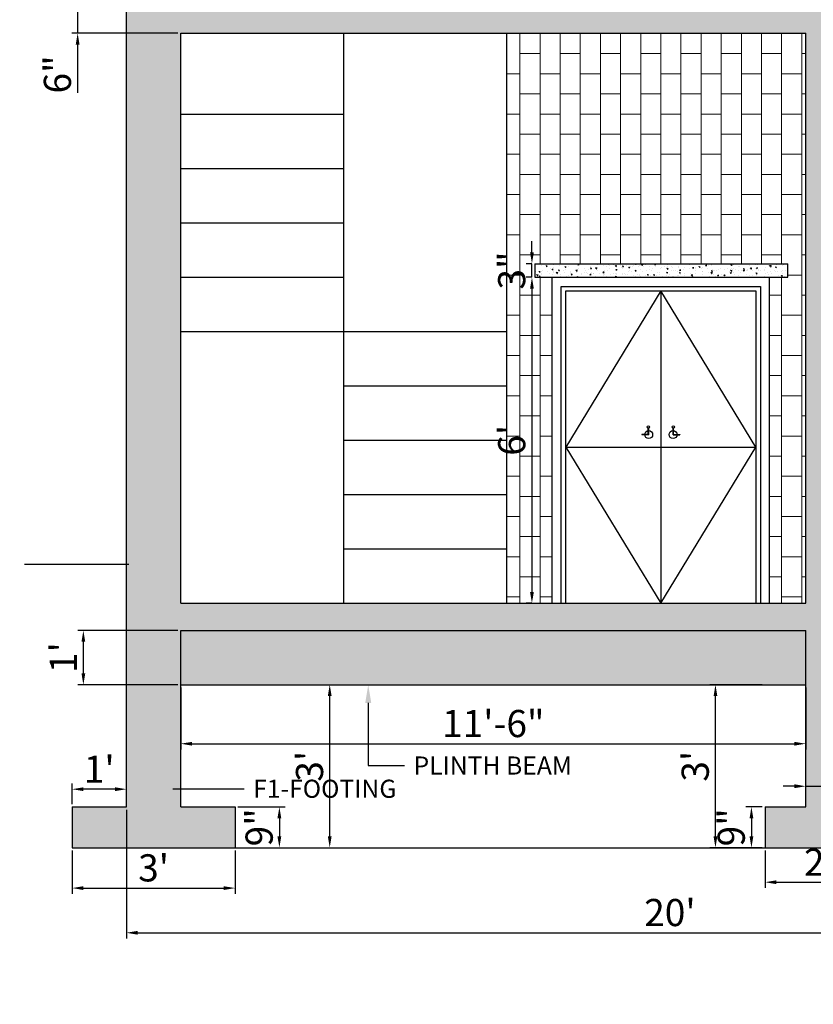
# Model space of a CAD drawing. Units: millimetres. Extents: x 20768 to 23556, y 50760 to 52704.
# Tile 3 of 36: x 20949 to 21124, y 51066 to 51283. Entities that reach past the tile are written whole.
import ezdxf
from ezdxf import colors
from ezdxf.entities.mleader import LeaderData, LeaderLine
from ezdxf.math import Vec2, Vec3

# ---------------------------------------------------------------- set-up
doc = ezdxf.new("R2010")
doc.units = ezdxf.units.MM
for name, color, linetype, lineweight in [('A-ANNO-DIMS', 2, 'Continuous', 18), ('A-ANNO-TEXT', 7, 'Continuous', 18), ('A-ELEV', 7, 'Continuous', 25), ('A-ELEV-PATT', 8, 'Continuous', 13), ('S-ANNO-DIMS', 2, 'Continuous', 18)]:
    doc.layers.add(name, color=color, linetype=linetype, lineweight=lineweight)
doc.styles.get("Standard").update_dxf_attribs({"font": 'arial.ttf'})
doc.dimstyles.new('ISO-25', dxfattribs={"dimtxt": 6, "dimasz": 2.5, "dimexe": 1.25, "dimexo": 0.625, "dimtad": 1, "dimdec": 0, "dimlunit": 3, "dimtxsty": 'Standard', "dimcen": 2.5, "dimadec": 0, "dimazin": 0, "dimtfac": 1, "dimtdec": 0, "dimtmove": 0, "dimatfit": 3, "dimfxl": 1, "dimarcsym": 0})
pattern_1 = [(140, (105.777, 340.6355), (0.23908628, 2.732770035), [0.28575, -3.14325]), (85, (105.777, 340.6355), (-2.86585268, -0.52865132), [0.2286, -2.51460876]), (190.4514447, (105.797, 340.8633), (-2.62676628, 2.20411871), [0.24285013, -2.67135367]), (136.1842, (105.015, 340.6355), (0.63063492, 4.06618561), [0.428625, -4.714875]), (186.635558, (105.0677, 340.9744), (-3.71139187, 3.561062), [0.36427535, -4.00703412]), (81.184151, (105.015, 340.6355), (-3.71139187, 3.561062), [0.3428995, -3.77189598]), (111, (105.2056, 341.0165), (1.53397797, 2.27421587), [0.28575, -3.14325]), (56, (105.2056, 341.0165), (-2.76281949, 0.92703043), [0.2286, -2.5146]), (161.451445, (105.3334, 341.206), (-1.22884153, 3.20124629), [0.24285013, -2.67134906]), (127.5, (105.7771, 340.6355), (-1.268325583, 0.046329049), [0, -2.48412, 0, -2.5527, 0, -2.524125]), (97.5, (105.7771, 340.6355), (-1.502708622, 1.002294938), [0, -1.45542, 0, -2.42697, 0, -0.962025]), (57.5, (105.7771, 339.7859), (0.08593116, 2.033858928), [0, -0.9525, 0, -2.9718, 0, -3.94335]), (47.5, (105.7771, 339.4049), (-0.381397365, 2.22193772), [0, -1.23825, 0, -1.97358, 0, -2.80035])]

# ---------------------------------------------------------------- blocks, each defined once
blk = doc.blocks.new('*D130')
at = {"layer": 'A-ANNO-DIMS', "color": 0, "lineweight": -2, "transparency": 16777216}
for p, q in [((20984.63, 51135.87), (20984.63, 51122.22)), ((21122.63, 51135.87), (21122.63, 51122.22)), ((20987.13, 51123.47), (21120.13, 51123.47))]:
    blk.add_line(p, q, dxfattribs=at)
at = {"layer": 'A-ANNO-DIMS', "color": 0, "transparency": 16777216}
for points in [[(20987.13, 51123.88), (20987.13, 51123.05), (20984.63, 51123.47)], [(21120.13, 51123.88), (21120.13, 51123.05), (21122.63, 51123.47)]]:
    blk.add_solid(points, dxfattribs=at)
at = {"layer": 'Defpoints', "color": 0, "transparency": 16777216}
for p in [(20984.63, 51136.5), (21122.63, 51136.5), (21122.63, 51123.47)]:
    blk.add_point(p, dxfattribs=at)
at = {"layer": 'A-ANNO-DIMS', "color": 0, "transparency": 16777216, "insert": (21053.63, 51127.15), "char_height": 6, "attachment_point": 5}
blk.add_mtext('11\'-6"', dxfattribs=at)
blk = doc.blocks.new('*D131')
at = {"layer": 'A-ANNO-DIMS', "color": 0, "lineweight": -2, "transparency": 16777216}
for p, q in [((20960.63, 51099.87), (20960.63, 51090.33)), ((20996.63, 51099.87), (20996.63, 51090.33)), ((20963.13, 51091.58), (20994.13, 51091.58))]:
    blk.add_line(p, q, dxfattribs=at)
at = {"layer": 'A-ANNO-DIMS', "color": 0, "transparency": 16777216}
for points in [[(20963.13, 51091.99), (20963.13, 51091.16), (20960.63, 51091.58)], [(20994.13, 51091.99), (20994.13, 51091.16), (20996.63, 51091.58)]]:
    blk.add_solid(points, dxfattribs=at)
at = {"layer": 'Defpoints', "color": 0, "transparency": 16777216}
for p in [(20960.63, 51100.5), (20996.63, 51100.5), (20996.63, 51091.58)]:
    blk.add_point(p, dxfattribs=at)
at = {"layer": 'A-ANNO-DIMS', "color": 0, "transparency": 16777216, "insert": (20978.63, 51095.27), "char_height": 6, "attachment_point": 5}
blk.add_mtext("3'", dxfattribs=at)
blk = doc.blocks.new('*D132')
at = {"layer": 'A-ANNO-DIMS', "color": 0, "lineweight": -2, "transparency": 16777216}
for p, q in [((20997.26, 51109.5), (21007.65, 51109.5)), ((21006.4, 51107), (21006.4, 51103)), ((20997.26, 51100.5), (21007.65, 51100.5))]:
    blk.add_line(p, q, dxfattribs=at)
at = {"layer": 'A-ANNO-DIMS', "color": 0, "transparency": 16777216}
for points in [[(21005.98, 51107), (21006.82, 51107), (21006.4, 51109.5)], [(21005.98, 51103), (21006.82, 51103), (21006.4, 51100.5)]]:
    blk.add_solid(points, dxfattribs=at)
at = {"layer": 'Defpoints', "color": 0, "transparency": 16777216}
for p in [(20996.63, 51109.5), (20996.63, 51100.5), (21006.4, 51100.5)]:
    blk.add_point(p, dxfattribs=at)
at = {"layer": 'A-ANNO-DIMS', "color": 0, "transparency": 16777216, "insert": (21002.71, 51105), "char_height": 6, "attachment_point": 5, "rotation": 90}
blk.add_mtext('9"', dxfattribs=at)
blk = doc.blocks.new('*D133')
at = {"layer": 'A-ANNO-DIMS', "color": 0, "lineweight": -2, "transparency": 16777216}
for p, q in [((20960.63, 51110.12), (20960.63, 51114.67)), ((20972.63, 51110.12), (20972.63, 51114.67)), ((20970.13, 51113.42), (20963.13, 51113.42))]:
    blk.add_line(p, q, dxfattribs=at)
at = {"layer": 'A-ANNO-DIMS', "color": 0, "transparency": 16777216}
for points in [[(20963.13, 51113.84), (20963.13, 51113.01), (20960.63, 51113.42)], [(20970.13, 51113.84), (20970.13, 51113.01), (20972.63, 51113.42)]]:
    blk.add_solid(points, dxfattribs=at)
at = {"layer": 'Defpoints', "color": 0, "transparency": 16777216}
for p in [(20960.63, 51113.42), (20960.63, 51109.5), (20972.63, 51109.5)]:
    blk.add_point(p, dxfattribs=at)
at = {"layer": 'A-ANNO-DIMS', "color": 0, "transparency": 16777216, "insert": (20966.63, 51117.06), "char_height": 6, "attachment_point": 5}
blk.add_mtext("1'", dxfattribs=at)
blk = doc.blocks.new('*D135')
at = {"layer": 'A-ANNO-DIMS', "color": 0, "lineweight": -2, "transparency": 16777216}
for p, q in [((21122.63, 51110.12), (21122.63, 51115.33)), ((21128.63, 51110.12), (21128.63, 51115.33)), ((21120.13, 51114.08), (21117.63, 51114.08)), ((21122.63, 51114.08), (21128.63, 51114.08)), ((21131.13, 51114.08), (21141.81, 51114.08))]:
    blk.add_line(p, q, dxfattribs=at)
at = {"layer": 'A-ANNO-DIMS', "color": 0, "transparency": 16777216}
for points in [[(21120.13, 51114.5), (21120.13, 51113.66), (21122.63, 51114.08)], [(21131.13, 51114.5), (21131.13, 51113.66), (21128.63, 51114.08)]]:
    blk.add_solid(points, dxfattribs=at)
at = {"layer": 'Defpoints', "color": 0, "transparency": 16777216}
for p in [(21128.63, 51114.08), (21122.63, 51109.5), (21128.63, 51109.5)]:
    blk.add_point(p, dxfattribs=at)
at = {"layer": 'A-ANNO-DIMS', "color": 0, "transparency": 16777216, "insert": (21137.72, 51117.77), "char_height": 6, "attachment_point": 5}
blk.add_mtext('6"', dxfattribs=at)
blk = doc.blocks.new('*D136')
at = {"layer": 'A-ANNO-DIMS', "color": 0, "lineweight": -2, "transparency": 16777216}
for p, q in [((21113.63, 51099.87), (21113.63, 51091.63)), ((21137.63, 51099.87), (21137.63, 51091.63)), ((21116.13, 51092.88), (21135.13, 51092.88))]:
    blk.add_line(p, q, dxfattribs=at)
at = {"layer": 'A-ANNO-DIMS', "color": 0, "transparency": 16777216}
for points in [[(21116.13, 51093.29), (21116.13, 51092.46), (21113.63, 51092.88)], [(21135.13, 51093.29), (21135.13, 51092.46), (21137.63, 51092.88)]]:
    blk.add_solid(points, dxfattribs=at)
at = {"layer": 'Defpoints', "color": 0, "transparency": 16777216}
for p in [(21113.63, 51100.5), (21137.63, 51100.5), (21137.63, 51092.88)]:
    blk.add_point(p, dxfattribs=at)
at = {"layer": 'A-ANNO-DIMS', "color": 0, "transparency": 16777216, "insert": (21125.63, 51096.52), "char_height": 6, "attachment_point": 5}
blk.add_mtext("2'", dxfattribs=at)
blk = doc.blocks.new('*D137')
at = {"layer": 'A-ANNO-DIMS', "color": 0, "lineweight": -2, "transparency": 16777216}
for p, q in [((21113.01, 51109.5), (21109.37, 51109.5)), ((21110.62, 51107), (21110.62, 51103)), ((21113.01, 51100.5), (21109.37, 51100.5))]:
    blk.add_line(p, q, dxfattribs=at)
at = {"layer": 'A-ANNO-DIMS', "color": 0, "transparency": 16777216}
for points in [[(21110.21, 51107), (21111.04, 51107), (21110.62, 51109.5)], [(21110.21, 51103), (21111.04, 51103), (21110.62, 51100.5)]]:
    blk.add_solid(points, dxfattribs=at)
at = {"layer": 'Defpoints', "color": 0, "transparency": 16777216}
for p in [(21113.63, 51109.5), (21110.62, 51100.5), (21113.63, 51100.5)]:
    blk.add_point(p, dxfattribs=at)
at = {"layer": 'A-ANNO-DIMS', "color": 0, "transparency": 16777216, "insert": (21106.94, 51105), "char_height": 6, "attachment_point": 5, "rotation": 90}
blk.add_mtext('9"', dxfattribs=at)
blk = doc.blocks.new('*D112')
at = {"layer": 'A-ANNO-DIMS', "color": 0, "lineweight": -2, "transparency": 16777216}
for p, q in [((20997.26, 51136.5), (21018.77, 51136.5)), ((21017.52, 51103), (21017.52, 51134)), ((20997.26, 51100.5), (21018.77, 51100.5))]:
    blk.add_line(p, q, dxfattribs=at)
at = {"layer": 'A-ANNO-DIMS', "color": 0, "transparency": 16777216}
for points in [[(21017.1, 51134), (21017.93, 51134), (21017.52, 51136.5)], [(21017.1, 51103), (21017.93, 51103), (21017.52, 51100.5)]]:
    blk.add_solid(points, dxfattribs=at)
at = {"layer": 'Defpoints', "color": 0, "transparency": 16777216}
for p in [(20996.63, 51136.5), (21017.52, 51136.5), (20996.63, 51100.5)]:
    blk.add_point(p, dxfattribs=at)
at = {"layer": 'A-ANNO-DIMS', "color": 0, "transparency": 16777216, "insert": (21013.83, 51118.5), "char_height": 6, "attachment_point": 5, "rotation": 90}
blk.add_mtext("3'", dxfattribs=at)
blk = doc.blocks.new('*D115')
at = {"layer": 'A-ANNO-DIMS', "color": 0, "lineweight": -2, "transparency": 16777216}
for p, q in [((20961.86, 51288.9), (20961.86, 51291.4)), ((20984.01, 51286.4), (20960.61, 51286.4)), ((20961.86, 51286.4), (20961.86, 51280.4)), ((20984.01, 51280.4), (20960.61, 51280.4)), ((20961.86, 51277.9), (20961.86, 51267.22))]:
    blk.add_line(p, q, dxfattribs=at)
at = {"layer": 'A-ANNO-DIMS', "color": 0, "transparency": 16777216}
for points in [[(20961.44, 51288.9), (20962.28, 51288.9), (20961.86, 51286.4)], [(20961.44, 51277.9), (20962.28, 51277.9), (20961.86, 51280.4)]]:
    blk.add_solid(points, dxfattribs=at)
at = {"layer": 'Defpoints', "color": 0, "transparency": 16777216}
for p in [(20984.63, 51286.4), (20961.86, 51280.4), (20984.63, 51280.4)]:
    blk.add_point(p, dxfattribs=at)
at = {"layer": 'A-ANNO-DIMS', "color": 0, "transparency": 16777216, "insert": (20958.17, 51271.31), "char_height": 6, "attachment_point": 5, "rotation": 90}
blk.add_mtext('6"', dxfattribs=at)
blk = doc.blocks.new('*D124')
at = {"layer": 'A-ANNO-DIMS', "color": 0, "lineweight": -2, "transparency": 16777216}
for p, q in [((21062.17, 51226.5), (21060.91, 51226.5)), ((21062.16, 51224), (21062.16, 51157)), ((21062.17, 51154.5), (21060.91, 51154.5))]:
    blk.add_line(p, q, dxfattribs=at)
at = {"layer": 'A-ANNO-DIMS', "color": 0, "transparency": 16777216}
for points in [[(21061.75, 51224), (21062.58, 51224), (21062.16, 51226.5)], [(21061.75, 51157), (21062.58, 51157), (21062.16, 51154.5)]]:
    blk.add_solid(points, dxfattribs=at)
at = {"layer": 'Defpoints', "color": 0, "transparency": 16777216}
for p in [(21062.79, 51226.5), (21062.16, 51154.5), (21062.79, 51154.5)]:
    blk.add_point(p, dxfattribs=at)
at = {"layer": 'A-ANNO-DIMS', "color": 0, "transparency": 16777216, "insert": (21058.48, 51190.5), "char_height": 6, "attachment_point": 5, "rotation": 90}
blk.add_mtext("6'", dxfattribs=at)
blk = doc.blocks.new('*D125')
at = {"layer": 'A-ANNO-DIMS', "color": 0, "lineweight": -2, "transparency": 16777216}
for p, q in [((21062.16, 51232), (21062.16, 51234.5)), ((21062.17, 51229.5), (21060.91, 51229.5)), ((21062.16, 51226.5), (21062.16, 51229.5)), ((21062.17, 51226.5), (21060.91, 51226.5)), ((21062.16, 51224), (21062.16, 51221.5))]:
    blk.add_line(p, q, dxfattribs=at)
at = {"layer": 'A-ANNO-DIMS', "color": 0, "transparency": 16777216}
for points in [[(21061.75, 51232), (21062.58, 51232), (21062.16, 51229.5)], [(21061.75, 51224), (21062.58, 51224), (21062.16, 51226.5)]]:
    blk.add_solid(points, dxfattribs=at)
at = {"layer": 'Defpoints', "color": 0, "transparency": 16777216}
for p in [(21062.16, 51229.5), (21062.79, 51229.5), (21062.79, 51226.5)]:
    blk.add_point(p, dxfattribs=at)
at = {"layer": 'A-ANNO-DIMS', "color": 0, "transparency": 16777216, "insert": (21058.47, 51228), "char_height": 6, "attachment_point": 5, "rotation": 90}
blk.add_mtext('3"', dxfattribs=at)
blk = doc.blocks.new('*D126')
at = {"layer": 'A-ANNO-DIMS', "color": 0, "lineweight": -2, "transparency": 16777216}
for p, q in [((20984.01, 51148.5), (20961.87, 51148.5)), ((20963.12, 51139), (20963.12, 51146)), ((20984.01, 51136.5), (20961.87, 51136.5))]:
    blk.add_line(p, q, dxfattribs=at)
at = {"layer": 'A-ANNO-DIMS', "color": 0, "transparency": 16777216}
for points in [[(20962.71, 51146), (20963.54, 51146), (20963.12, 51148.5)], [(20962.71, 51139), (20963.54, 51139), (20963.12, 51136.5)]]:
    blk.add_solid(points, dxfattribs=at)
at = {"layer": 'Defpoints', "color": 0, "transparency": 16777216}
for p in [(20963.12, 51148.5), (20984.63, 51148.5), (20984.63, 51136.5)]:
    blk.add_point(p, dxfattribs=at)
at = {"layer": 'A-ANNO-DIMS', "color": 0, "transparency": 16777216, "insert": (20959.49, 51142.5), "char_height": 6, "attachment_point": 5, "rotation": 90}
blk.add_mtext("1'", dxfattribs=at)
blk = doc.blocks.new('*D128')
at = {"layer": 'A-ANNO-DIMS', "color": 0, "lineweight": -2, "transparency": 16777216}
for p, q in [((21113.01, 51136.5), (21101.43, 51136.5)), ((21102.68, 51103), (21102.68, 51134)), ((21113.01, 51100.5), (21101.43, 51100.5))]:
    blk.add_line(p, q, dxfattribs=at)
at = {"layer": 'A-ANNO-DIMS', "color": 0, "transparency": 16777216}
for points in [[(21102.27, 51134), (21103.1, 51134), (21102.68, 51136.5)], [(21102.27, 51103), (21103.1, 51103), (21102.68, 51100.5)]]:
    blk.add_solid(points, dxfattribs=at)
at = {"layer": 'Defpoints', "color": 0, "transparency": 16777216}
for p in [(21102.68, 51136.5), (21113.63, 51136.5), (21113.63, 51100.5)]:
    blk.add_point(p, dxfattribs=at)
at = {"layer": 'A-ANNO-DIMS', "color": 0, "transparency": 16777216, "insert": (21098.99, 51118.5), "char_height": 6, "attachment_point": 5, "rotation": 90}
blk.add_mtext("3'", dxfattribs=at)
blk = doc.blocks.new('*D111')
at = {"layer": 'A-ANNO-DIMS', "color": 0, "lineweight": -2, "transparency": 16777216}
for p, q in [((20972.63, 51108.87), (20972.63, 51080.46)), ((21212.63, 51108.87), (21212.63, 51080.46)), ((20975.13, 51081.71), (21210.13, 51081.71))]:
    blk.add_line(p, q, dxfattribs=at)
at = {"layer": 'A-ANNO-DIMS', "color": 0, "transparency": 16777216}
for points in [[(20975.13, 51082.13), (20975.13, 51081.29), (20972.63, 51081.71)], [(21210.13, 51082.13), (21210.13, 51081.29), (21212.63, 51081.71)]]:
    blk.add_solid(points, dxfattribs=at)
at = {"layer": 'Defpoints', "color": 0, "transparency": 16777216}
for p in [(20972.63, 51109.5), (21212.63, 51109.5), (21212.63, 51081.71)]:
    blk.add_point(p, dxfattribs=at)
at = {"layer": 'A-ANNO-DIMS', "color": 0, "transparency": 16777216, "insert": (21092.63, 51085.4), "char_height": 6, "attachment_point": 5}
blk.add_mtext("20'", dxfattribs=at)
blk = doc.blocks.new('*D229')
at = {"layer": 'Defpoints', "color": 0, "transparency": 16777216}
for p in [(20963.6, 51532.3), (20960.63, 51100.5), (21253.63, 51100.5)]:
    blk.add_point(p, dxfattribs=at)
at = {"layer": 'S-ANNO-DIMS', "color": 0, "lineweight": -2, "transparency": 16777216}
for p, q in [((20964.22, 51532.3), (21254.88, 51532.3)), ((21253.63, 51529.8), (21253.63, 51103)), ((20961.26, 51100.5), (21254.88, 51100.5))]:
    blk.add_line(p, q, dxfattribs=at)
at = {"layer": 'S-ANNO-DIMS', "color": 0, "transparency": 16777216}
for points in [[(21253.22, 51529.8), (21254.05, 51529.8), (21253.63, 51532.3)], [(21253.22, 51103), (21254.05, 51103), (21253.63, 51100.5)]]:
    blk.add_solid(points, dxfattribs=at)
at = {"layer": 'S-ANNO-DIMS', "color": 0, "transparency": 16777216, "insert": (21249.94, 51316.4), "char_height": 6, "attachment_point": 5, "rotation": 90}
blk.add_mtext('36\'-0"', dxfattribs=at)

msp = doc.modelspace()

# ---------------------------------------------------------------- hatches: boundary and pattern name
at = {"layer": 'A-ELEV-PATT'}
h = msp.add_hatch(dxfattribs=at)
h.set_pattern_fill('AR-CONC', color=256, scale=0.015, angle=90)
h.set_pattern_definition(pattern_1)
h.paths.add_polyline_path([(21212.63, 51490.3), (21200.63, 51490.3), (21200.63, 51418.3), (21128.63, 51418.3), (21128.63, 51490.3), (21122.63, 51490.3), (21122.63, 51418.3), (20972.63, 51418.3), (20972.63, 51109.5), (20960.63, 51109.5), (20960.63, 51100.5), (20996.63, 51100.5), (20996.63, 51109.5), (20984.63, 51109.5), (20984.63, 51148.5), (21122.63, 51148.5), (21122.63, 51109.5), (21113.63, 51109.5), (21113.63, 51100.5), (21137.63, 51100.5), (21137.63, 51109.5), (21128.63, 51109.5), (21128.63, 51148.5), (21212.63, 51148.5)])
h.paths.add_polyline_path([(21122.63, 51280.4), (21122.63, 51154.5), (20984.63, 51154.5), (20984.63, 51280.4)], flags=16)
h.paths.add_polyline_path([(21122.63, 51286.4), (20984.63, 51286.4), (20984.63, 51412.3), (21122.63, 51412.3)], flags=16)
h.paths.add_polyline_path([(21128.63, 51280.4), (21200.63, 51280.4), (21200.63, 51154.5), (21128.63, 51154.5)], flags=16)
h.paths.add_polyline_path([(21128.63, 51286.4), (21128.63, 51412.3), (21200.63, 51412.3), (21200.63, 51286.4)], flags=16)
h.paths.add_polyline_path([(21062.79, 51358.4), (21062.79, 51361.4), (21118.63, 51361.4), (21118.63, 51358.4)], flags=0)
h.paths.add_polyline_path([(21111.63, 51320.9), (21090.63, 51286.4), (21069.63, 51320.9), (21069.63, 51355.4), (21111.63, 51355.4)], flags=0)
h.paths.add_polyline_path([(21069.63, 51320.9), (21090.63, 51355.4), (21111.63, 51320.9)], flags=0)
h.paths.add_polyline_path([(21136.63, 51320.9), (21136.63, 51368), (21167.33, 51368), (21167.33, 51320.9)], flags=0)
h.paths.add_polyline_path([(21138.63, 51322.9), (21138.63, 51350.9), (21165.33, 51350.9), (21165.33, 51322.9)], flags=0)
h.paths.add_polyline_path([(21140.63, 51324.9), (21140.63, 51348.9), (21150.98, 51348.9), (21150.98, 51324.9)], flags=0)
h.paths.add_polyline_path([(21136.63, 51236.1), (21167.33, 51236.1), (21167.33, 51189), (21136.63, 51189)], flags=0)
h.paths.add_polyline_path([(21152.98, 51324.9), (21152.98, 51348.9), (21163.33, 51348.9), (21163.33, 51324.9)], flags=0)
h.paths.add_polyline_path([(21094.84, 51323.58), (21094.21, 51323.58, -0.960515), (21092.46, 51323.65, -0.414214), (21093.33, 51324.52), (21093.33, 51325.09, -0.357901), (21093.11, 51325.35, -1), (21093.66, 51325.35, -0.34824), (21093.45, 51325.09), (21093.45, 51324.51, -0.376216), (21094.21, 51323.65), (21094.84, 51323.65)], flags=0)
h.paths.add_polyline_path([(21138.63, 51234.1), (21165.33, 51234.1), (21165.33, 51221), (21138.63, 51221)], flags=0)
h.paths.add_polyline_path([(21118.63, 51229.5), (21118.63, 51226.5), (21062.79, 51226.5), (21062.79, 51229.5)], flags=0)
h.paths.add_polyline_path([(21087.06, 51323.58), (21086.42, 51323.58), (21086.42, 51323.65), (21087.06, 51323.65, -0.376216), (21087.82, 51324.51), (21087.82, 51325.09, -0.34824), (21087.61, 51325.35, -1), (21088.15, 51325.35, -0.357901), (21087.94, 51325.09), (21087.94, 51324.52, -0.414214), (21088.81, 51323.65, -0.960515)], flags=0)
h.paths.add_polyline_path([(21111.63, 51223.5), (21111.63, 51189), (21090.63, 51154.5), (21069.63, 51189), (21069.63, 51223.5)], flags=0)
h.paths.add_polyline_path([(21138.63, 51219), (21165.33, 51219), (21165.33, 51191), (21138.63, 51191)], flags=0)
h.paths.add_polyline_path([(21140.63, 51217), (21150.98, 51217), (21150.98, 51193), (21140.63, 51193)], flags=0)
h.paths.add_polyline_path([(21056.63, 51166.5), (21020.63, 51166.5), (21020.63, 51214.5), (21056.63, 51214.5)], flags=0)
h.paths.add_polyline_path([(21056.63, 51298.4), (21020.63, 51298.4), (21020.63, 51346.4), (21056.63, 51346.4)], flags=0)
h.paths.add_polyline_path([(21090.63, 51223.5), (21111.63, 51189), (21069.63, 51189)], flags=0)
h.paths.add_polyline_path([(21138.63, 51352.9), (21138.63, 51366), (21165.33, 51366), (21165.33, 51352.9)], flags=0)
h.paths.add_polyline_path([(21152.98, 51217), (21163.33, 51217), (21163.33, 51193), (21152.98, 51193)], flags=0)
h.paths.add_polyline_path([(21093.66, 51193.45, -0.34824), (21093.45, 51193.19), (21093.45, 51192.61, -0.376216), (21094.21, 51191.75), (21094.84, 51191.75), (21094.84, 51191.68), (21094.21, 51191.68, -0.960515), (21092.46, 51191.75, -0.414214), (21093.33, 51192.62), (21093.33, 51193.19, -0.357901), (21093.11, 51193.45, -1)], flags=0)
h.paths.add_polyline_path([(21088.15, 51193.45, -0.357901), (21087.94, 51193.19), (21087.94, 51192.62, -0.414214), (21088.81, 51191.75, -0.960515), (21087.06, 51191.68), (21086.42, 51191.68), (21086.42, 51191.75), (21087.06, 51191.75, -0.376216), (21087.82, 51192.61), (21087.82, 51193.19, -0.34824), (21087.61, 51193.45, -1)], flags=0)
h = msp.add_hatch(dxfattribs=at)
h.set_pattern_fill('BRICK', color=256, scale=0.7, angle=90)
h.set_pattern_definition([(90, (105.777, 340.6355), (-4.445, 3e-16), []), (180, (105.777, 340.6355), (-1e-15, -8.89), [4.445, -4.445]), (180, (105.777, 345.0805), (-1e-15, -8.89), [-4.445, 4.445])])
h.paths.add_polyline_path([(21122.63, 51280.4), (21056.63, 51280.4), (21056.63, 51154.5), (21066.63, 51154.5), (21066.63, 51226.5), (21062.79, 51226.5), (21062.79, 51229.5), (21118.63, 51229.5), (21118.63, 51226.5), (21114.63, 51226.5), (21114.63, 51154.5), (21122.63, 51154.5)])
h = msp.add_hatch(dxfattribs=at)
h.set_pattern_fill('AR-CONC', color=256, scale=0.015, angle=90)
h.paths.add_polyline_path([(21118.63, 51229.5), (21062.79, 51229.5), (21062.79, 51226.5), (21118.63, 51226.5)])
h = msp.add_hatch(dxfattribs=at)
h.set_pattern_fill('AR-CONC', color=256, scale=8)
h.paths.add_polyline_path([(21106.86, 51149.66), (21094.86, 51149.66), (21094.86, 51077.66), (21022.86, 51077.66), (21022.86, 51149.66), (21016.86, 51149.66), (21016.86, 51077.66), (20866.86, 51077.66), (20866.86, 50768.86), (20854.86, 50768.86), (20854.86, 50759.86), (20890.86, 50759.86), (20890.86, 50768.86), (20878.86, 50768.86), (20878.86, 50807.86), (21016.86, 50807.86), (21016.86, 50768.86), (21007.86, 50768.86), (21007.86, 50759.86), (21031.86, 50759.86), (21031.86, 50768.86), (21022.86, 50768.86), (21022.86, 50807.86), (21094.86, 50807.86), (21094.86, 50768.86), (21082.86, 50768.86), (21082.86, 50759.86), (21118.86, 50759.86), (21118.86, 50768.86), (21106.86, 50768.86)])
h.paths.add_polyline_path([(21022.86, 50939.76), (21094.86, 50939.76), (21094.86, 50813.86), (21022.86, 50813.86)], flags=16)
h.paths.add_polyline_path([(21016.86, 50939.76), (21016.86, 50813.86), (20878.86, 50813.86), (20878.86, 50939.76)], flags=16)
h.paths.add_polyline_path([(21022.86, 50945.76), (21022.86, 51071.66), (21094.86, 51071.66), (21094.86, 50945.76)], flags=16)
h.paths.add_polyline_path([(21016.86, 50945.76), (20878.86, 50945.76), (20878.86, 51071.66), (21016.86, 51071.66)], flags=16)
h.paths.add_polyline_path([(20957.01, 51017.76), (20957.01, 51020.76), (21012.86, 51020.76), (21012.86, 51017.76)], flags=0)
h.paths.add_polyline_path([(21005.86, 50980.26), (20984.86, 50945.76), (20963.86, 50980.26), (20963.86, 51014.76), (21005.86, 51014.76)], flags=0)
h.paths.add_polyline_path([(20963.86, 50980.26), (20984.86, 51014.76), (21005.86, 50980.26)], flags=0)
h.paths.add_polyline_path([(21030.86, 50980.26), (21030.86, 51027.36), (21061.56, 51027.36), (21061.56, 50980.26)], flags=0)
h.paths.add_polyline_path([(21032.86, 50982.26), (21032.86, 51010.26), (21059.56, 51010.26), (21059.56, 50982.26)], flags=0)
h.paths.add_polyline_path([(21034.86, 50984.26), (21034.86, 51008.26), (21045.21, 51008.26), (21045.21, 50984.26)], flags=0)
h.paths.add_polyline_path([(21030.86, 50895.46), (21061.56, 50895.46), (21061.56, 50848.36), (21030.86, 50848.36)], flags=0)
h.paths.add_polyline_path([(21032.86, 50893.46), (21059.56, 50893.46), (21059.56, 50880.36), (21032.86, 50880.36)], flags=0)
h.paths.add_polyline_path([(21047.21, 50984.26), (21047.21, 51008.26), (21057.56, 51008.26), (21057.56, 50984.26)], flags=0)
h.paths.add_polyline_path([(20989.07, 50982.94), (20988.43, 50982.94, -0.960515), (20986.68, 50983.01, -0.414214), (20987.56, 50983.89), (20987.56, 50984.45, -0.357901), (20987.34, 50984.72, -1), (20987.88, 50984.72, -0.34824), (20987.67, 50984.45), (20987.67, 50983.88, -0.376216), (20988.43, 50983.01), (20989.07, 50983.01)], flags=0)
h.paths.add_polyline_path([(21012.86, 50888.86), (21012.86, 50885.86), (20957.01, 50885.86), (20957.01, 50888.86)], flags=0)
h.paths.add_polyline_path([(20981.29, 50982.94), (20980.65, 50982.94), (20980.65, 50983.01), (20981.28, 50983.01, -0.376216), (20982.04, 50983.88), (20982.04, 50984.45, -0.34824), (20981.83, 50984.72, -1), (20982.38, 50984.72, -0.357901), (20982.16, 50984.45), (20982.16, 50983.89, -0.414214), (20983.04, 50983.01, -0.960515)], flags=0)
h.paths.add_polyline_path([(21005.86, 50882.86), (21005.86, 50848.36), (20984.86, 50813.86), (20963.86, 50848.36), (20963.86, 50882.86)], flags=0)
h.paths.add_polyline_path([(21032.86, 50878.36), (21059.56, 50878.36), (21059.56, 50850.36), (21032.86, 50850.36)], flags=0)
h.paths.add_polyline_path([(21034.86, 50876.36), (21045.21, 50876.36), (21045.21, 50852.36), (21034.86, 50852.36)], flags=0)
h.paths.add_polyline_path([(20984.86, 50882.86), (21005.86, 50848.36), (20963.86, 50848.36)], flags=0)
h.paths.add_polyline_path([(20950.86, 50825.86), (20914.86, 50825.86), (20914.86, 50873.86), (20950.86, 50873.86)], flags=0)
h.paths.add_polyline_path([(20950.86, 50957.76), (20914.86, 50957.76), (20914.86, 51005.76), (20950.86, 51005.76)], flags=0)
h.paths.add_polyline_path([(21047.21, 50876.36), (21057.56, 50876.36), (21057.56, 50852.36), (21047.21, 50852.36)], flags=0)
h.paths.add_polyline_path([(21032.86, 51012.26), (21032.86, 51025.36), (21059.56, 51025.36), (21059.56, 51012.26)], flags=0)
h.paths.add_polyline_path([(20987.88, 50852.82, -0.34824), (20987.67, 50852.55), (20987.67, 50851.98, -0.376216), (20988.43, 50851.11), (20989.07, 50851.11), (20989.07, 50851.04), (20988.43, 50851.04, -0.960515), (20986.68, 50851.11, -0.414214), (20987.56, 50851.99), (20987.56, 50852.55, -0.357901), (20987.34, 50852.82, -1)], flags=0)
h.paths.add_polyline_path([(20982.38, 50852.82, -0.357901), (20982.16, 50852.55), (20982.16, 50851.99, -0.414214), (20983.04, 50851.11, -0.960515), (20981.29, 50851.04), (20980.65, 50851.04), (20980.65, 50851.11), (20981.28, 50851.11, -0.376216), (20982.04, 50851.98), (20982.04, 50852.55, -0.34824), (20981.83, 50852.82, -1)], flags=0)
h = msp.add_hatch(dxfattribs=at)
h.set_pattern_fill('AR-CONC', color=256, scale=0.015, angle=90)
h.set_pattern_definition(pattern_1)
h.paths.add_polyline_path([(21122.63, 51148.5), (20984.63, 51148.5), (20984.63, 51136.5), (21122.63, 51136.5)])

# ---------------------------------------------------------------- linework, layer by layer
at = {"layer": 'A-ELEV'}
for p, q in [((20972.63, 51109.5), (20972.63, 51526.3)), ((20984.63, 51154.5), (20984.63, 51280.4)), ((20984.63, 51280.4), (21122.63, 51280.4)), ((21020.63, 51154.5), (21020.63, 51280.4)), ((21056.63, 51154.5), (21056.63, 51280.4)), ((21122.63, 51154.5), (21122.63, 51280.4)), ((20984.63, 51262.5), (21020.63, 51262.5)), ((20984.63, 51250.5), (21020.63, 51250.5)), ((20984.63, 51238.5), (21020.63, 51238.5)), ((21062.79, 51229.5), (21118.63, 51229.5)), ((21062.79, 51229.5), (21062.79, 51226.5)), ((21118.63, 51226.5), (21118.63, 51229.5)), ((20984.63, 51226.5), (21020.63, 51226.5)), ((21062.79, 51226.5), (21118.63, 51226.5)), ((21066.63, 51154.5), (21066.63, 51226.5)), ((21114.63, 51154.5), (21114.63, 51226.5)), ((21090.63, 51223.5), (21090.63, 51154.5)), ((20984.63, 51214.5), (21056.63, 51214.5)), ((21020.63, 51202.5), (21056.63, 51202.5)), ((21087.82, 51191.75), (21087.82, 51193.19)), ((21087.94, 51191.68), (21087.94, 51193.19)), ((21093.33, 51191.68), (21093.33, 51193.19)), ((21093.45, 51191.75), (21093.45, 51193.19)), ((21087.82, 51191.75), (21086.42, 51191.75)), ((21086.42, 51191.75), (21086.42, 51191.68)), ((21087.94, 51191.68), (21086.42, 51191.68)), ((21093.33, 51191.68), (21094.84, 51191.68)), ((21093.45, 51191.75), (21094.84, 51191.75)), ((21094.84, 51191.75), (21094.84, 51191.68)), ((21020.63, 51190.5), (21056.63, 51190.5)), ((21069.63, 51189), (21111.63, 51189)), ((21020.63, 51178.5), (21056.63, 51178.5)), ((21020.63, 51166.5), (21056.63, 51166.5)), ((20984.63, 51154.5), (21122.63, 51154.5)), ((20984.63, 51109.5), (20984.63, 51148.5)), ((20984.63, 51148.5), (21122.63, 51148.5)), ((21122.63, 51109.5), (21122.63, 51148.5)), ((20984.63, 51136.5), (21122.63, 51136.5)), ((20960.63, 51109.5), (20972.63, 51109.5)), ((20960.63, 51109.5), (20960.63, 51100.5)), ((20984.63, 51109.5), (20996.63, 51109.5)), ((20996.63, 51109.5), (20996.63, 51100.5)), ((21113.63, 51109.5), (21122.63, 51109.5)), ((21113.63, 51109.5), (21113.63, 51100.5)), ((20960.63, 51100.5), (20996.63, 51100.5)), ((21113.63, 51100.5), (21137.63, 51100.5))]:
    msp.add_line(p, q, dxfattribs=at)
for points in [[(21068.63, 51154.5), (21068.63, 51224.5), (21112.63, 51224.5), (21112.63, 51154.5)], [(21069.63, 51154.5), (21069.63, 51223.5), (21111.63, 51223.5), (21111.63, 51154.5)]]:
    msp.add_lwpolyline(points, dxfattribs=at)
msp.add_lwpolyline([(21111.63, 51189), (21090.63, 51223.5), (21069.63, 51189), (21090.63, 51154.5)], close=True, dxfattribs=at)
for centre, radius in [((21087.88, 51193.45), 0.272), ((21093.39, 51193.45), 0.272), ((21087.94, 51191.75), 0.877), ((21093.33, 51191.75), 0.877)]:
    msp.add_circle(centre, radius, dxfattribs=at)

# ---------------------------------------------------------------- dimensions: what is measured, and where the dimension line sits
at = {"layer": 'A-ANNO-DIMS'}
for base, p1, p2, picture, middle in [((20961.86, 51280.4), (20984.63, 51286.4), (20984.63, 51280.4), '*D115', (20958.17, 51271.31)), ((21062.16, 51154.5), (21062.79, 51226.5), (21062.79, 51154.5), '*D124', (21058.48, 51190.5)), ((20963.12, 51148.5), (20984.63, 51136.5), (20984.63, 51148.5), '*D126', (20959.49, 51142.5)), ((21017.52, 51136.5), (20996.63, 51100.5), (20996.63, 51136.5), '*D112', (21013.83, 51118.5)), ((21102.68, 51136.5), (21113.63, 51100.5), (21113.63, 51136.5), '*D128', (21098.99, 51118.5)), ((21006.4, 51100.5), (20996.63, 51109.5), (20996.63, 51100.5), '*D132', (21002.71, 51105)), ((21110.62, 51100.5), (21113.63, 51109.5), (21113.63, 51100.5), '*D137', (21106.94, 51105))]:
    dim = msp.add_linear_dim(base=base, p1=p1, p2=p2, angle=90, dimstyle='ISO-25', override={"dimclrd": 0, "dimclre": 0, "dimclrt": 0}, dxfattribs=at)
    dim.commit()
    dim.dimension.update_dxf_attribs({"geometry": picture, "text_midpoint": middle})
dim = msp.add_linear_dim(base=(21062.16, 51229.5), p1=(21062.79, 51226.5), p2=(21062.79, 51229.5), angle=90, dimstyle='ISO-25', override={"dimclrd": 0, "dimclre": 0, "dimclrt": 0}, dxfattribs=at)
dim.commit()
dim.dimension.update_dxf_attribs({"geometry": '*D125', "text_midpoint": (21062.16, 51228), "dimtype": 160})
for base, p1, p2, picture, middle in [((21122.63, 51123.47), (20984.63, 51136.5), (21122.63, 51136.5), '*D130', (21053.63, 51127.15)), ((20960.63, 51113.42), (20972.63, 51109.5), (20960.63, 51109.5), '*D133', (20966.63, 51117.06)), ((21128.63, 51114.08), (21122.63, 51109.5), (21128.63, 51109.5), '*D135', (21137.72, 51117.77)), ((21212.63, 51081.71), (20972.63, 51109.5), (21212.63, 51109.5), '*D111', (21092.63, 51085.4)), ((20996.63, 51091.58), (20960.63, 51100.5), (20996.63, 51100.5), '*D131', (20978.63, 51095.27)), ((21137.63, 51092.88), (21113.63, 51100.5), (21137.63, 51100.5), '*D136', (21125.63, 51096.52))]:
    dim = msp.add_linear_dim(base=base, p1=p1, p2=p2, dimstyle='ISO-25', override={"dimclrd": 0, "dimclre": 0, "dimclrt": 0}, dxfattribs=at)
    dim.commit()
    dim.dimension.update_dxf_attribs({"geometry": picture, "text_midpoint": middle})
at = {"layer": 'S-ANNO-DIMS'}
dim = msp.add_linear_dim(base=(21253.63, 51100.5), p1=(20963.6, 51532.3), p2=(20960.63, 51100.5), angle=90, dimstyle='ISO-25', override={"dimdec": 1, "dimlfac": 1, "dimrnd": 0, "dimzin": 1, "dimdsep": 46, "dimlunit": 4, "dimfrac": 2}, dxfattribs=at)
dim.commit()
dim.dimension.update_dxf_attribs({"geometry": '*D229', "text_midpoint": (21249.94, 51316.4)})

# ---------------------------------------------------------------- leaders
at = {"layer": 'A-ANNO-TEXT'}
ml = msp.add_multileader_mtext('Standard', dxfattribs=at)
ml.set_content('C1-COLUMN', color=256)
ml.set_leader_properties()
ml.build(insert=Vec2(0, 0))
ctx = ml.context
ctx.base_point, ctx.char_height, ctx.plane_origin = Vec3(20873.04, 51163.09), 9, Vec3(20977.17, 51163.09)
ctx.text_align_type = 2
notes = []
notes.append((ctx, [(0, (1, 1, 0), (20958.12, 51163.09), (-1, 0), 8, [(0, [(20977.17, 51163.09)], 0, [])])]))
ctx.mtext.insert, ctx.mtext.alignment, ctx.mtext.flow_direction = Vec3(20948.12, 51167.67), 3, 5
ml = msp.add_multileader_mtext('Standard', dxfattribs=at)
ml.set_content('PLINTH BEAM', color=256)
ml.set_leader_properties()
ml.build(insert=Vec2(0, 0))
ctx = ml.context
ctx.base_point, ctx.plane_origin = Vec3(21034.02, 51118.65), Vec3(21026.02, 51136.5)
notes.append((ctx, [(0, (1, 1, 0), (21026.02, 51118.65), (1, 0), 8, [(0, [(21026.02, 51136.5)], 0, [])])]))
ctx.mtext.insert, ctx.mtext.flow_direction = Vec3(21036.02, 51120.65), 5
ml = msp.add_multileader_mtext('Standard', dxfattribs=at)
ml.set_content('F1-FOOTING', color=256)
ml.set_leader_properties()
ml.build(insert=Vec2(0, 0))
ctx = ml.context
ctx.base_point, ctx.plane_origin = Vec3(20998.61, 51113.49), Vec3(20978.85, 51113.49)
notes.append((ctx, [(0, (1, 1, 0), (20990.61, 51113.49), (1, 0), 8, [(0, [(20978.85, 51113.49)], 0, [])])]))
ctx.mtext.insert, ctx.mtext.flow_direction = Vec3(21000.61, 51115.52), 5
for ctx, leaders in notes:
    for number, flags, end, landing, length, lines in leaders:
        leader = LeaderData()
        leader.index, (leader.has_last_leader_line, leader.has_dogleg_vector, leader.attachment_direction) = number, flags
        leader.last_leader_point, leader.dogleg_vector, leader.dogleg_length = Vec3(end), Vec3(landing), length
        for number, points, colour, breaks in lines:
            line = LeaderLine()
            line.index, line.vertices, line.color, line.breaks = number, Vec3.list(points), colors.encode_raw_color(colour), breaks
            leader.lines.append(line)
        ctx.leaders.append(leader)

doc.saveas('drawing.dxf')
